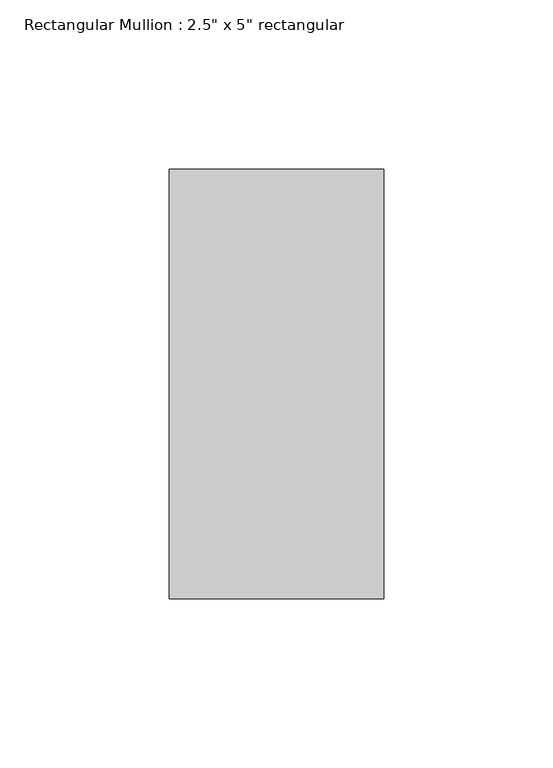
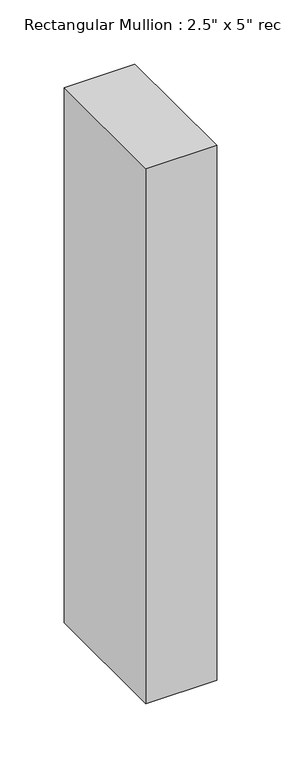
"""IFC4 building model written with IfcOpenShell, lengths in millimetres: member geometry."""

from ifc_helpers import new_model, si_unit, frame, origin, place, context, project, spatial, polyline, outline, extrude, source, transform, mapped, element, save


def member_7fd687a9(model_context):
    return source(origin(), model_context, "Body", "SweptSolid", [
        extrude(outline(polyline([(0.0, 63.5), (0.0, -63.5), (-63.5, -63.5), (-63.5, 63.5), (0.0, 63.5)])), frame((0.0, 0.0, -508.0), z_axis=(0.0, 0.0, 1.0), x_axis=(1.0, 0.0, 0.0)), (0.0, 0.0, 1.0), 508.0),
    ])


if __name__ == "__main__":
    model = new_model("IFC4")
    model_context = context("Model", 3, world=origin())
    ifc_project = project(units=[si_unit("LENGTHUNIT", "METRE", prefix="MILLI")], contexts=[model_context])
    site = spatial("IfcSite", under=ifc_project)
    building = spatial("IfcBuilding", under=site)
    placement = place(None, origin())
    member_shape = member_7fd687a9(model_context)
    element("IfcMember", 1, ObjectType="Rectangular Mullion : 2.5\" x 5\" rectangular", at=placement, inside=building, context=model_context, shape_type="MappedRepresentation", body=[
        mapped(member_shape, transform((0.0, 0.0, 0.0), x_axis=(1.0, 0.0, 0.0), y_axis=(0.0, 1.0, 0.0), z_axis=(0.0, 0.0, 1.0))),
    ])
    save(model, "model.ifc")

# Revit data of these elements
# Type "Rectangular Mullion : 2.5\" x 5\" rectangular"
#   built-in parameter 1007304 = 0.416667 (stored number, unit not read)
#   built-in parameter 1007301 = 0.104167 (stored number, unit not read)
#   built-in parameter 1007300 = 0.104167 (stored number, unit not read)
# Element 1 (IfcMember, "Rectangular Mullion : 2.5\" x 5\" rectangular")
#   Materials on its faces: "Aluminum"
# Materials
#   "Aluminum": class "Metal", colour RGB 247 247 247, transparency 0, Description = "Aluminum 6061", Cost = 0
